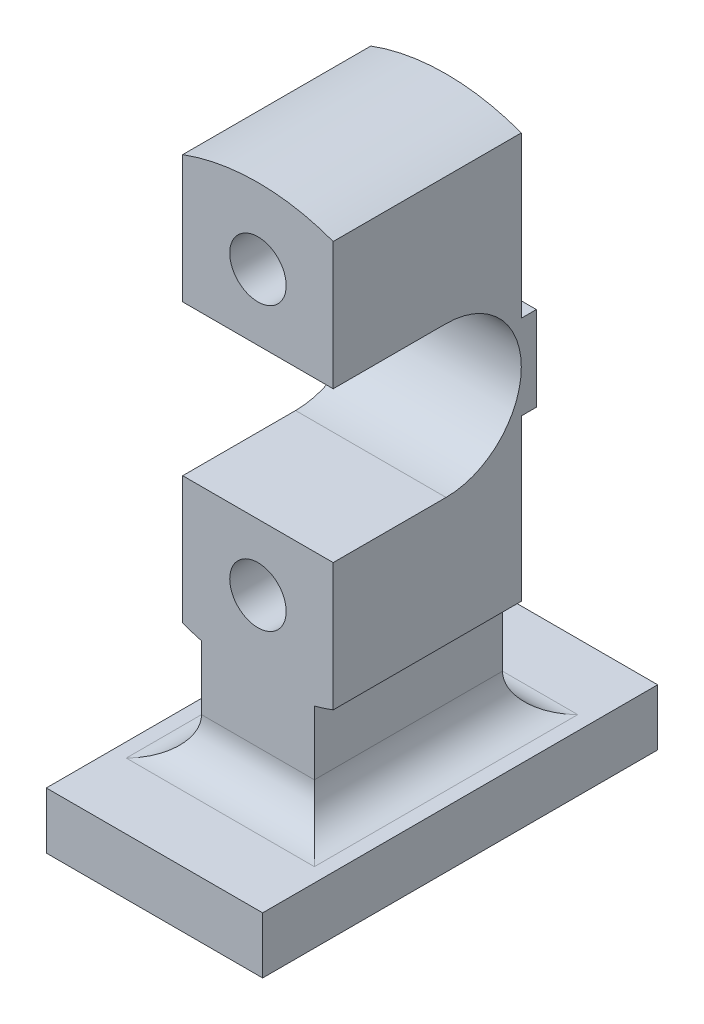
ISO-10303-21;
HEADER;
FILE_DESCRIPTION(('STEP AP214'),'2;1');
FILE_NAME('part.step','',(''),(''),'','','');
FILE_SCHEMA(('AUTOMOTIVE_DESIGN { 1 0 10303 214 1 1 1 1 }'));
ENDSEC;
DATA;
#1=APPLICATION_CONTEXT('core data for automotive mechanical design processes');
#2=APPLICATION_PROTOCOL_DEFINITION('international standard','automotive_design',2000,#1);
#3=PRODUCT_CONTEXT('',#1,'mechanical');
#4=PRODUCT('Part','Part','',(#3));
#5=PRODUCT_RELATED_PRODUCT_CATEGORY('part','',(#4));
#6=PRODUCT_DEFINITION_FORMATION('','',#4);
#7=PRODUCT_DEFINITION_CONTEXT('part definition',#1,'design');
#8=PRODUCT_DEFINITION('design','',#6,#7);
#9=PRODUCT_DEFINITION_SHAPE('','',#8);
#10=(LENGTH_UNIT() NAMED_UNIT(*) SI_UNIT(.MILLI.,.METRE.));
#11=(NAMED_UNIT(*) PLANE_ANGLE_UNIT() SI_UNIT($,.RADIAN.));
#12=(NAMED_UNIT(*) SI_UNIT($,.STERADIAN.) SOLID_ANGLE_UNIT());
#13=UNCERTAINTY_MEASURE_WITH_UNIT(LENGTH_MEASURE(1.E-05),#10,'distance_accuracy_value','');
#14=(GEOMETRIC_REPRESENTATION_CONTEXT(3) GLOBAL_UNCERTAINTY_ASSIGNED_CONTEXT((#13)) GLOBAL_UNIT_ASSIGNED_CONTEXT((#10,
#11,#12)) REPRESENTATION_CONTEXT('',''));
#15=CARTESIAN_POINT('',(0.,0.,0.));
#16=DIRECTION('',(0.,0.,1.));
#17=DIRECTION('',(1.,0.,0.));
#18=AXIS2_PLACEMENT_3D('',#15,#16,#17);
#19=CARTESIAN_POINT('',(0.,0.,50.));
#20=DIRECTION('',(0.,0.,-1.));
#21=DIRECTION('',(-1.,0.,0.));
#22=AXIS2_PLACEMENT_3D('',#19,#20,#21);
#23=PLANE('',#22);
#24=CARTESIAN_POINT('',(0.,-75.,50.));
#25=DIRECTION('',(0.,0.,1.));
#26=DIRECTION('',(-1.,0.,0.));
#27=AXIS2_PLACEMENT_3D('',#24,#25,#26);
#28=CIRCLE('',#27,15.);
#29=CARTESIAN_POINT('',(-15.,-75.,50.));
#30=VERTEX_POINT('',#29);
#31=EDGE_CURVE('E317',#30,#30,#28,.T.);
#32=ORIENTED_EDGE('',*,*,#31,.F.);
#33=EDGE_LOOP('',(#32));
#34=FACE_BOUND('',#33,.T.);
#35=DIRECTION('',(0.,1.,0.));
#36=VECTOR('',#35,1.);
#37=CARTESIAN_POINT('',(40.,-107.819293264239,50.));
#38=LINE('',#37,#36);
#39=CARTESIAN_POINT('',(40.,-107.819293264239,50.));
#40=VERTEX_POINT('',#39);
#41=CARTESIAN_POINT('',(40.,-40.,50.));
#42=VERTEX_POINT('',#41);
#43=EDGE_CURVE('E213',#40,#42,#38,.T.);
#44=ORIENTED_EDGE('',*,*,#43,.T.);
#45=DIRECTION('',(1.,0.,0.));
#46=VECTOR('',#45,1.);
#47=CARTESIAN_POINT('',(-168.062484748657,-40.,50.));
#48=LINE('',#47,#46);
#49=CARTESIAN_POINT('',(-40.,-40.,50.));
#50=VERTEX_POINT('',#49);
#51=EDGE_CURVE('E210',#50,#42,#48,.T.);
#52=ORIENTED_EDGE('',*,*,#51,.F.);
#53=DIRECTION('',(0.,-1.,0.));
#54=VECTOR('',#53,1.);
#55=CARTESIAN_POINT('',(-40.,-107.819293264239,50.));
#56=LINE('',#55,#54);
#57=CARTESIAN_POINT('',(-40.0000000000001,-107.819293264239,50.));
#58=VERTEX_POINT('',#57);
#59=EDGE_CURVE('E329',#50,#58,#56,.T.);
#60=ORIENTED_EDGE('',*,*,#59,.T.);
#61=CARTESIAN_POINT('',(0.,0.,50.));
#62=DIRECTION('',(0.,0.,1.));
#63=DIRECTION('',(1.,0.,0.));
#64=AXIS2_PLACEMENT_3D('',#61,#62,#63);
#65=CIRCLE('',#64,115.);
#66=CARTESIAN_POINT('',(-30.,-111.018016555873,50.));
#67=VERTEX_POINT('',#66);
#68=EDGE_CURVE('E335',#58,#67,#65,.T.);
#69=ORIENTED_EDGE('',*,*,#68,.T.);
#70=DIRECTION('',(0.,-1.,0.));
#71=VECTOR('',#70,1.);
#72=CARTESIAN_POINT('',(-30.,-111.018016555873,50.));
#73=LINE('',#72,#71);
#74=CARTESIAN_POINT('',(-30.,-145.,50.));
#75=VERTEX_POINT('',#74);
#76=EDGE_CURVE('E331',#67,#75,#73,.T.);
#77=ORIENTED_EDGE('',*,*,#76,.T.);
#78=DIRECTION('',(1.,0.,0.));
#79=VECTOR('',#78,1.);
#80=CARTESIAN_POINT('',(0.,-145.,50.));
#81=LINE('',#80,#79);
#82=CARTESIAN_POINT('',(30.,-145.,50.));
#83=VERTEX_POINT('',#82);
#84=EDGE_CURVE('E48',#75,#83,#81,.T.);
#85=ORIENTED_EDGE('',*,*,#84,.T.);
#86=DIRECTION('',(0.,1.,0.));
#87=VECTOR('',#86,1.);
#88=CARTESIAN_POINT('',(30.,-111.018016555873,50.));
#89=LINE('',#88,#87);
#90=CARTESIAN_POINT('',(30.,-111.018016555873,50.));
#91=VERTEX_POINT('',#90);
#92=EDGE_CURVE('E220',#83,#91,#89,.T.);
#93=ORIENTED_EDGE('',*,*,#92,.T.);
#94=CARTESIAN_POINT('',(0.,0.,50.));
#95=DIRECTION('',(0.,0.,1.));
#96=DIRECTION('',(1.,0.,0.));
#97=AXIS2_PLACEMENT_3D('',#94,#95,#96);
#98=CIRCLE('',#97,115.);
#99=EDGE_CURVE('E212',#91,#40,#98,.T.);
#100=ORIENTED_EDGE('',*,*,#99,.T.);
#101=EDGE_LOOP('',(#44,#52,#60,#69,#77,#85,#93,#100));
#102=FACE_BOUND('',#101,.T.);
#103=ADVANCED_FACE('F39',(#34,#102),#23,.F.);
#104=CARTESIAN_POINT('',(0.,0.,-50.));
#105=DIRECTION('',(0.,0.,-1.));
#106=DIRECTION('',(-1.,0.,0.));
#107=AXIS2_PLACEMENT_3D('',#104,#105,#106);
#108=PLANE('',#107);
#109=DIRECTION('',(1.,0.,0.));
#110=VECTOR('',#109,1.);
#111=CARTESIAN_POINT('',(-85.7055795281058,22.5,-50.));
#112=LINE('',#111,#110);
#113=CARTESIAN_POINT('',(-40.,22.5,-50.));
#114=VERTEX_POINT('',#113);
#115=CARTESIAN_POINT('',(40.,22.5,-50.));
#116=VERTEX_POINT('',#115);
#117=EDGE_CURVE('E409',#114,#116,#112,.T.);
#118=ORIENTED_EDGE('',*,*,#117,.F.);
#119=DIRECTION('',(0.,-1.,0.));
#120=VECTOR('',#119,1.);
#121=CARTESIAN_POINT('',(-40.,-107.819293264239,-50.));
#122=LINE('',#121,#120);
#123=CARTESIAN_POINT('',(-40.,107.819293264239,-50.));
#124=VERTEX_POINT('',#123);
#125=EDGE_CURVE('E227',#124,#114,#122,.T.);
#126=ORIENTED_EDGE('',*,*,#125,.F.);
#127=CARTESIAN_POINT('',(0.,0.,-50.));
#128=DIRECTION('',(0.,0.,1.));
#129=DIRECTION('',(-1.,0.,0.));
#130=AXIS2_PLACEMENT_3D('',#127,#128,#129);
#131=CIRCLE('',#130,115.);
#132=CARTESIAN_POINT('',(40.,107.819293264239,-50.));
#133=VERTEX_POINT('',#132);
#134=EDGE_CURVE('E222',#133,#124,#131,.T.);
#135=ORIENTED_EDGE('',*,*,#134,.F.);
#136=DIRECTION('',(0.,1.,0.));
#137=VECTOR('',#136,1.);
#138=CARTESIAN_POINT('',(40.,-107.819293264239,-50.));
#139=LINE('',#138,#137);
#140=EDGE_CURVE('E236',#116,#133,#139,.T.);
#141=ORIENTED_EDGE('',*,*,#140,.F.);
#142=EDGE_LOOP('',(#118,#126,#135,#141));
#143=FACE_BOUND('',#142,.T.);
#144=CARTESIAN_POINT('',(0.,75.,-50.));
#145=DIRECTION('',(0.,0.,1.));
#146=DIRECTION('',(1.,0.,0.));
#147=AXIS2_PLACEMENT_3D('',#144,#145,#146);
#148=CIRCLE('',#147,15.);
#149=CARTESIAN_POINT('',(15.,75.,-50.));
#150=VERTEX_POINT('',#149);
#151=EDGE_CURVE('E325',#150,#150,#148,.T.);
#152=ORIENTED_EDGE('',*,*,#151,.T.);
#153=EDGE_LOOP('',(#152));
#154=FACE_BOUND('',#153,.T.);
#155=ADVANCED_FACE('F450',(#143,#154),#108,.T.);
#156=CARTESIAN_POINT('',(-40.,107.819293264239,50.));
#157=VERTEX_POINT('',#156);
#158=CARTESIAN_POINT('',(-40.,40.,50.));
#159=VERTEX_POINT('',#158);
#160=EDGE_CURVE('E206',#157,#159,#56,.T.);
#161=ORIENTED_EDGE('',*,*,#160,.T.);
#162=DIRECTION('',(1.,0.,0.));
#163=VECTOR('',#162,1.);
#164=CARTESIAN_POINT('',(-168.062484748657,40.,50.));
#165=LINE('',#164,#163);
#166=CARTESIAN_POINT('',(40.,40.,50.));
#167=VERTEX_POINT('',#166);
#168=EDGE_CURVE('E192',#159,#167,#165,.T.);
#169=ORIENTED_EDGE('',*,*,#168,.T.);
#170=CARTESIAN_POINT('',(40.,107.819293264239,50.));
#171=VERTEX_POINT('',#170);
#172=EDGE_CURVE('E204',#167,#171,#38,.T.);
#173=ORIENTED_EDGE('',*,*,#172,.T.);
#174=CARTESIAN_POINT('',(0.,0.,50.));
#175=DIRECTION('',(0.,0.,1.));
#176=DIRECTION('',(-1.,0.,0.));
#177=AXIS2_PLACEMENT_3D('',#174,#175,#176);
#178=CIRCLE('',#177,115.);
#179=EDGE_CURVE('E244',#171,#157,#178,.T.);
#180=ORIENTED_EDGE('',*,*,#179,.T.);
#181=EDGE_LOOP('',(#161,#169,#173,#180));
#182=FACE_BOUND('',#181,.T.);
#183=CARTESIAN_POINT('',(0.,75.,50.));
#184=DIRECTION('',(0.,0.,1.));
#185=DIRECTION('',(1.,0.,0.));
#186=AXIS2_PLACEMENT_3D('',#183,#184,#185);
#187=CIRCLE('',#186,15.);
#188=CARTESIAN_POINT('',(15.,75.,50.));
#189=VERTEX_POINT('',#188);
#190=EDGE_CURVE('E223',#189,#189,#187,.T.);
#191=ORIENTED_EDGE('',*,*,#190,.F.);
#192=EDGE_LOOP('',(#191));
#193=FACE_BOUND('',#192,.T.);
#194=ADVANCED_FACE('F203',(#182,#193),#23,.F.);
#195=DIRECTION('',(1.,0.,0.));
#196=VECTOR('',#195,1.);
#197=CARTESIAN_POINT('',(-85.7055795281058,-22.5,-50.));
#198=LINE('',#197,#196);
#199=CARTESIAN_POINT('',(-40.,-22.5,-50.));
#200=VERTEX_POINT('',#199);
#201=CARTESIAN_POINT('',(40.,-22.5,-50.));
#202=VERTEX_POINT('',#201);
#203=EDGE_CURVE('E389',#200,#202,#198,.T.);
#204=ORIENTED_EDGE('',*,*,#203,.T.);
#205=CARTESIAN_POINT('',(40.,-107.819293264239,-50.));
#206=VERTEX_POINT('',#205);
#207=EDGE_CURVE('E239',#206,#202,#139,.T.);
#208=ORIENTED_EDGE('',*,*,#207,.F.);
#209=CARTESIAN_POINT('',(0.,0.,-50.));
#210=DIRECTION('',(0.,0.,1.));
#211=DIRECTION('',(1.,0.,0.));
#212=AXIS2_PLACEMENT_3D('',#209,#210,#211);
#213=CIRCLE('',#212,115.);
#214=CARTESIAN_POINT('',(30.,-111.018016555873,-50.));
#215=VERTEX_POINT('',#214);
#216=EDGE_CURVE('E237',#215,#206,#213,.T.);
#217=ORIENTED_EDGE('',*,*,#216,.F.);
#218=DIRECTION('',(0.,1.,0.));
#219=VECTOR('',#218,1.);
#220=CARTESIAN_POINT('',(30.,-111.018016555873,-50.));
#221=LINE('',#220,#219);
#222=CARTESIAN_POINT('',(30.,-145.,-50.));
#223=VERTEX_POINT('',#222);
#224=EDGE_CURVE('E235',#223,#215,#221,.T.);
#225=ORIENTED_EDGE('',*,*,#224,.F.);
#226=DIRECTION('',(1.,0.,0.));
#227=VECTOR('',#226,1.);
#228=CARTESIAN_POINT('',(-30.,-145.,-50.));
#229=LINE('',#228,#227);
#230=CARTESIAN_POINT('',(-30.,-145.,-50.));
#231=VERTEX_POINT('',#230);
#232=EDGE_CURVE('E268',#223,#231,#229,.F.);
#233=ORIENTED_EDGE('',*,*,#232,.T.);
#234=DIRECTION('',(0.,-1.,0.));
#235=VECTOR('',#234,1.);
#236=CARTESIAN_POINT('',(-30.,-111.018016555873,-50.));
#237=LINE('',#236,#235);
#238=CARTESIAN_POINT('',(-30.,-111.018016555873,-50.));
#239=VERTEX_POINT('',#238);
#240=EDGE_CURVE('E233',#239,#231,#237,.T.);
#241=ORIENTED_EDGE('',*,*,#240,.F.);
#242=CARTESIAN_POINT('',(0.,0.,-50.));
#243=DIRECTION('',(0.,0.,1.));
#244=DIRECTION('',(1.,0.,0.));
#245=AXIS2_PLACEMENT_3D('',#242,#243,#244);
#246=CIRCLE('',#245,115.);
#247=CARTESIAN_POINT('',(-40.0000000000001,-107.819293264239,-50.));
#248=VERTEX_POINT('',#247);
#249=EDGE_CURVE('E226',#248,#239,#246,.T.);
#250=ORIENTED_EDGE('',*,*,#249,.F.);
#251=EDGE_CURVE('E221',#200,#248,#122,.T.);
#252=ORIENTED_EDGE('',*,*,#251,.F.);
#253=EDGE_LOOP('',(#204,#208,#217,#225,#233,#241,#250,#252));
#254=FACE_BOUND('',#253,.T.);
#255=CARTESIAN_POINT('',(0.,-75.,-50.));
#256=DIRECTION('',(0.,0.,1.));
#257=DIRECTION('',(-1.,0.,0.));
#258=AXIS2_PLACEMENT_3D('',#255,#256,#257);
#259=CIRCLE('',#258,15.);
#260=CARTESIAN_POINT('',(-15.,-75.,-50.));
#261=VERTEX_POINT('',#260);
#262=EDGE_CURVE('E318',#261,#261,#259,.T.);
#263=ORIENTED_EDGE('',*,*,#262,.T.);
#264=EDGE_LOOP('',(#263));
#265=FACE_BOUND('',#264,.T.);
#266=ADVANCED_FACE('F378',(#254,#265),#108,.T.);
#267=CARTESIAN_POINT('',(0.,0.,50.));
#268=DIRECTION('',(0.,0.,-1.));
#269=DIRECTION('',(-1.,0.,0.));
#270=AXIS2_PLACEMENT_3D('',#267,#268,#269);
#271=CYLINDRICAL_SURFACE('',#270,115.);
#272=ORIENTED_EDGE('',*,*,#134,.T.);
#273=DIRECTION('',(0.,0.,-1.));
#274=VECTOR('',#273,1.);
#275=CARTESIAN_POINT('',(-40.,107.819293264239,50.));
#276=LINE('',#275,#274);
#277=EDGE_CURVE('E258',#157,#124,#276,.T.);
#278=ORIENTED_EDGE('',*,*,#277,.F.);
#279=ORIENTED_EDGE('',*,*,#179,.F.);
#280=DIRECTION('',(0.,0.,-1.));
#281=VECTOR('',#280,1.);
#282=CARTESIAN_POINT('',(40.,107.819293264239,50.));
#283=LINE('',#282,#281);
#284=EDGE_CURVE('E211',#171,#133,#283,.T.);
#285=ORIENTED_EDGE('',*,*,#284,.T.);
#286=EDGE_LOOP('',(#272,#278,#279,#285));
#287=FACE_BOUND('',#286,.T.);
#288=ADVANCED_FACE('F461',(#287),#271,.T.);
#289=CARTESIAN_POINT('',(-40.,-107.819293264239,50.));
#290=DIRECTION('',(1.,0.,0.));
#291=DIRECTION('',(0.,0.,-1.));
#292=AXIS2_PLACEMENT_3D('',#289,#290,#291);
#293=PLANE('',#292);
#294=ORIENTED_EDGE('',*,*,#59,.F.);
#295=DIRECTION('',(0.,0.,1.));
#296=VECTOR('',#295,1.);
#297=CARTESIAN_POINT('',(-40.,-40.,-10.));
#298=LINE('',#297,#296);
#299=CARTESIAN_POINT('',(-40.,-40.,-10.));
#300=VERTEX_POINT('',#299);
#301=EDGE_CURVE('E362',#300,#50,#298,.T.);
#302=ORIENTED_EDGE('',*,*,#301,.F.);
#303=CARTESIAN_POINT('',(-40.,0.,-9.99999999999999));
#304=DIRECTION('',(1.,0.,0.));
#305=DIRECTION('',(0.,0.,-1.));
#306=AXIS2_PLACEMENT_3D('',#303,#304,#305);
#307=CIRCLE('',#306,40.);
#308=CARTESIAN_POINT('',(-40.,40.,-10.));
#309=VERTEX_POINT('',#308);
#310=EDGE_CURVE('E396',#309,#300,#307,.F.);
#311=ORIENTED_EDGE('',*,*,#310,.F.);
#312=DIRECTION('',(0.,0.,-1.));
#313=VECTOR('',#312,1.);
#314=CARTESIAN_POINT('',(-40.,40.,-10.));
#315=LINE('',#314,#313);
#316=EDGE_CURVE('E399',#159,#309,#315,.T.);
#317=ORIENTED_EDGE('',*,*,#316,.F.);
#318=ORIENTED_EDGE('',*,*,#160,.F.);
#319=ORIENTED_EDGE('',*,*,#277,.T.);
#320=ORIENTED_EDGE('',*,*,#125,.T.);
#321=DIRECTION('',(0.,0.,-1.));
#322=VECTOR('',#321,1.);
#323=CARTESIAN_POINT('',(-40.,22.5,-50.));
#324=LINE('',#323,#322);
#325=CARTESIAN_POINT('',(-40.,22.5,-58.));
#326=VERTEX_POINT('',#325);
#327=EDGE_CURVE('E401',#114,#326,#324,.T.);
#328=ORIENTED_EDGE('',*,*,#327,.T.);
#329=DIRECTION('',(0.,-1.,0.));
#330=VECTOR('',#329,1.);
#331=CARTESIAN_POINT('',(-40.,22.5,-58.));
#332=LINE('',#331,#330);
#333=CARTESIAN_POINT('',(-40.,-22.5,-58.));
#334=VERTEX_POINT('',#333);
#335=EDGE_CURVE('E406',#326,#334,#332,.T.);
#336=ORIENTED_EDGE('',*,*,#335,.T.);
#337=DIRECTION('',(0.,0.,1.));
#338=VECTOR('',#337,1.);
#339=CARTESIAN_POINT('',(-40.,-22.5,-50.));
#340=LINE('',#339,#338);
#341=EDGE_CURVE('E280',#334,#200,#340,.T.);
#342=ORIENTED_EDGE('',*,*,#341,.T.);
#343=ORIENTED_EDGE('',*,*,#251,.T.);
#344=DIRECTION('',(0.,0.,-1.));
#345=VECTOR('',#344,1.);
#346=CARTESIAN_POINT('',(-40.0000000000001,-107.819293264239,50.));
#347=LINE('',#346,#345);
#348=EDGE_CURVE('E251',#58,#248,#347,.T.);
#349=ORIENTED_EDGE('',*,*,#348,.F.);
#350=EDGE_LOOP('',(#294,#302,#311,#317,#318,#319,#320,#328,#336,#342,#343,#349));
#351=FACE_BOUND('',#350,.T.);
#352=ADVANCED_FACE('F356',(#351),#293,.F.);
#353=CARTESIAN_POINT('',(0.,0.,50.));
#354=DIRECTION('',(0.,0.,-1.));
#355=DIRECTION('',(-1.,0.,0.));
#356=AXIS2_PLACEMENT_3D('',#353,#354,#355);
#357=CYLINDRICAL_SURFACE('',#356,115.);
#358=ORIENTED_EDGE('',*,*,#249,.T.);
#359=DIRECTION('',(0.,0.,-1.));
#360=VECTOR('',#359,1.);
#361=CARTESIAN_POINT('',(-30.,-111.018016555873,50.));
#362=LINE('',#361,#360);
#363=EDGE_CURVE('E246',#67,#239,#362,.T.);
#364=ORIENTED_EDGE('',*,*,#363,.F.);
#365=ORIENTED_EDGE('',*,*,#68,.F.);
#366=ORIENTED_EDGE('',*,*,#348,.T.);
#367=EDGE_LOOP('',(#358,#364,#365,#366));
#368=FACE_BOUND('',#367,.T.);
#369=ADVANCED_FACE('F366',(#368),#357,.T.);
#370=CARTESIAN_POINT('',(-30.,-111.018016555873,50.));
#371=DIRECTION('',(1.,0.,0.));
#372=DIRECTION('',(0.,1.,0.));
#373=AXIS2_PLACEMENT_3D('',#370,#371,#372);
#374=PLANE('',#373);
#375=ORIENTED_EDGE('',*,*,#240,.T.);
#376=DIRECTION('',(0.,0.,-1.));
#377=VECTOR('',#376,1.);
#378=CARTESIAN_POINT('',(-30.,-145.,50.));
#379=LINE('',#378,#377);
#380=EDGE_CURVE('E271',#231,#75,#379,.F.);
#381=ORIENTED_EDGE('',*,*,#380,.T.);
#382=ORIENTED_EDGE('',*,*,#76,.F.);
#383=ORIENTED_EDGE('',*,*,#363,.T.);
#384=EDGE_LOOP('',(#375,#381,#382,#383));
#385=FACE_BOUND('',#384,.T.);
#386=ADVANCED_FACE('F387',(#385),#374,.F.);
#387=CARTESIAN_POINT('',(30.,-111.018016555873,50.));
#388=DIRECTION('',(-1.,0.,0.));
#389=DIRECTION('',(0.,-1.,0.));
#390=AXIS2_PLACEMENT_3D('',#387,#388,#389);
#391=PLANE('',#390);
#392=ORIENTED_EDGE('',*,*,#92,.F.);
#393=DIRECTION('',(0.,0.,-1.));
#394=VECTOR('',#393,1.);
#395=CARTESIAN_POINT('',(30.,-145.,50.));
#396=LINE('',#395,#394);
#397=EDGE_CURVE('E11',#83,#223,#396,.T.);
#398=ORIENTED_EDGE('',*,*,#397,.T.);
#399=ORIENTED_EDGE('',*,*,#224,.T.);
#400=DIRECTION('',(0.,0.,-1.));
#401=VECTOR('',#400,1.);
#402=CARTESIAN_POINT('',(30.,-111.018016555873,50.));
#403=LINE('',#402,#401);
#404=EDGE_CURVE('E249',#91,#215,#403,.T.);
#405=ORIENTED_EDGE('',*,*,#404,.F.);
#406=EDGE_LOOP('',(#392,#398,#399,#405));
#407=FACE_BOUND('',#406,.T.);
#408=ADVANCED_FACE('F342',(#407),#391,.F.);
#409=CARTESIAN_POINT('',(0.,0.,50.));
#410=DIRECTION('',(0.,0.,-1.));
#411=DIRECTION('',(-1.,0.,0.));
#412=AXIS2_PLACEMENT_3D('',#409,#410,#411);
#413=CYLINDRICAL_SURFACE('',#412,115.);
#414=ORIENTED_EDGE('',*,*,#216,.T.);
#415=DIRECTION('',(0.,0.,-1.));
#416=VECTOR('',#415,1.);
#417=CARTESIAN_POINT('',(40.,-107.819293264239,50.));
#418=LINE('',#417,#416);
#419=EDGE_CURVE('E241',#40,#206,#418,.T.);
#420=ORIENTED_EDGE('',*,*,#419,.F.);
#421=ORIENTED_EDGE('',*,*,#99,.F.);
#422=ORIENTED_EDGE('',*,*,#404,.T.);
#423=EDGE_LOOP('',(#414,#420,#421,#422));
#424=FACE_BOUND('',#423,.T.);
#425=ADVANCED_FACE('F350',(#424),#413,.T.);
#426=CARTESIAN_POINT('',(40.,-107.819293264239,50.));
#427=DIRECTION('',(-1.,0.,0.));
#428=DIRECTION('',(0.,0.,1.));
#429=AXIS2_PLACEMENT_3D('',#426,#427,#428);
#430=PLANE('',#429);
#431=CARTESIAN_POINT('',(40.,0.,-9.99999999999999));
#432=DIRECTION('',(1.,0.,0.));
#433=DIRECTION('',(0.,0.,-1.));
#434=AXIS2_PLACEMENT_3D('',#431,#432,#433);
#435=CIRCLE('',#434,40.);
#436=CARTESIAN_POINT('',(40.,-40.,-10.));
#437=VERTEX_POINT('',#436);
#438=CARTESIAN_POINT('',(40.,40.,-9.99999999999999));
#439=VERTEX_POINT('',#438);
#440=EDGE_CURVE('E57',#437,#439,#435,.T.);
#441=ORIENTED_EDGE('',*,*,#440,.F.);
#442=DIRECTION('',(0.,0.,-1.));
#443=VECTOR('',#442,1.);
#444=CARTESIAN_POINT('',(40.,-40.,-10.));
#445=LINE('',#444,#443);
#446=EDGE_CURVE('E197',#42,#437,#445,.T.);
#447=ORIENTED_EDGE('',*,*,#446,.F.);
#448=ORIENTED_EDGE('',*,*,#43,.F.);
#449=ORIENTED_EDGE('',*,*,#419,.T.);
#450=ORIENTED_EDGE('',*,*,#207,.T.);
#451=DIRECTION('',(0.,0.,-1.));
#452=VECTOR('',#451,1.);
#453=CARTESIAN_POINT('',(40.,-22.5,-50.));
#454=LINE('',#453,#452);
#455=CARTESIAN_POINT('',(40.,-22.5,-58.));
#456=VERTEX_POINT('',#455);
#457=EDGE_CURVE('E391',#202,#456,#454,.T.);
#458=ORIENTED_EDGE('',*,*,#457,.T.);
#459=DIRECTION('',(0.,1.,0.));
#460=VECTOR('',#459,1.);
#461=CARTESIAN_POINT('',(40.,22.5,-58.));
#462=LINE('',#461,#460);
#463=CARTESIAN_POINT('',(40.,22.5,-58.));
#464=VERTEX_POINT('',#463);
#465=EDGE_CURVE('E398',#456,#464,#462,.T.);
#466=ORIENTED_EDGE('',*,*,#465,.T.);
#467=DIRECTION('',(0.,0.,1.));
#468=VECTOR('',#467,1.);
#469=CARTESIAN_POINT('',(40.,22.5,-50.));
#470=LINE('',#469,#468);
#471=EDGE_CURVE('E61',#464,#116,#470,.T.);
#472=ORIENTED_EDGE('',*,*,#471,.T.);
#473=ORIENTED_EDGE('',*,*,#140,.T.);
#474=ORIENTED_EDGE('',*,*,#284,.F.);
#475=ORIENTED_EDGE('',*,*,#172,.F.);
#476=DIRECTION('',(0.,0.,1.));
#477=VECTOR('',#476,1.);
#478=CARTESIAN_POINT('',(40.,40.,-10.));
#479=LINE('',#478,#477);
#480=EDGE_CURVE('E188',#439,#167,#479,.T.);
#481=ORIENTED_EDGE('',*,*,#480,.F.);
#482=EDGE_LOOP('',(#441,#447,#448,#449,#450,#458,#466,#472,#473,#474,#475,#481));
#483=FACE_BOUND('',#482,.T.);
#484=ADVANCED_FACE('F207',(#483),#430,.F.);
#485=CARTESIAN_POINT('',(0.,75.,50.));
#486=DIRECTION('',(0.,0.,-1.));
#487=DIRECTION('',(-1.,0.,0.));
#488=AXIS2_PLACEMENT_3D('',#485,#486,#487);
#489=CYLINDRICAL_SURFACE('',#488,15.);
#490=ORIENTED_EDGE('',*,*,#190,.T.);
#491=EDGE_LOOP('',(#490));
#492=FACE_BOUND('',#491,.T.);
#493=ORIENTED_EDGE('',*,*,#151,.F.);
#494=EDGE_LOOP('',(#493));
#495=FACE_BOUND('',#494,.T.);
#496=ADVANCED_FACE('F475',(#492,#495),#489,.F.);
#497=CARTESIAN_POINT('',(0.,-75.,50.));
#498=DIRECTION('',(0.,0.,-1.));
#499=DIRECTION('',(-1.,0.,0.));
#500=AXIS2_PLACEMENT_3D('',#497,#498,#499);
#501=CYLINDRICAL_SURFACE('',#500,15.);
#502=ORIENTED_EDGE('',*,*,#31,.T.);
#503=EDGE_LOOP('',(#502));
#504=FACE_BOUND('',#503,.T.);
#505=ORIENTED_EDGE('',*,*,#262,.F.);
#506=EDGE_LOOP('',(#505));
#507=FACE_BOUND('',#506,.T.);
#508=ADVANCED_FACE('F619',(#504,#507),#501,.F.);
#509=CARTESIAN_POINT('',(57.5,-195.,-105.));
#510=DIRECTION('',(-1.,0.,0.));
#511=DIRECTION('',(0.,0.,1.));
#512=AXIS2_PLACEMENT_3D('',#509,#510,#511);
#513=PLANE('',#512);
#514=DIRECTION('',(0.,0.,1.));
#515=VECTOR('',#514,1.);
#516=CARTESIAN_POINT('',(57.5,-165.,-105.));
#517=LINE('',#516,#515);
#518=CARTESIAN_POINT('',(57.5,-165.,-105.));
#519=VERTEX_POINT('',#518);
#520=CARTESIAN_POINT('',(57.5,-165.,105.));
#521=VERTEX_POINT('',#520);
#522=EDGE_CURVE('E283',#519,#521,#517,.T.);
#523=ORIENTED_EDGE('',*,*,#522,.T.);
#524=DIRECTION('',(0.,1.,0.));
#525=VECTOR('',#524,1.);
#526=CARTESIAN_POINT('',(57.5,-195.,105.));
#527=LINE('',#526,#525);
#528=CARTESIAN_POINT('',(57.5,-195.,105.));
#529=VERTEX_POINT('',#528);
#530=EDGE_CURVE('E312',#529,#521,#527,.T.);
#531=ORIENTED_EDGE('',*,*,#530,.F.);
#532=DIRECTION('',(0.,0.,1.));
#533=VECTOR('',#532,1.);
#534=CARTESIAN_POINT('',(57.5,-195.,-105.));
#535=LINE('',#534,#533);
#536=CARTESIAN_POINT('',(57.5,-195.,-105.));
#537=VERTEX_POINT('',#536);
#538=EDGE_CURVE('E308',#537,#529,#535,.T.);
#539=ORIENTED_EDGE('',*,*,#538,.F.);
#540=DIRECTION('',(0.,1.,0.));
#541=VECTOR('',#540,1.);
#542=CARTESIAN_POINT('',(57.5,-195.,-105.));
#543=LINE('',#542,#541);
#544=EDGE_CURVE('E307',#537,#519,#543,.T.);
#545=ORIENTED_EDGE('',*,*,#544,.T.);
#546=EDGE_LOOP('',(#523,#531,#539,#545));
#547=FACE_BOUND('',#546,.T.);
#548=ADVANCED_FACE('F428',(#547),#513,.F.);
#549=CARTESIAN_POINT('',(-57.5,-195.,105.));
#550=DIRECTION('',(0.,0.,-1.));
#551=DIRECTION('',(-1.,0.,0.));
#552=AXIS2_PLACEMENT_3D('',#549,#550,#551);
#553=PLANE('',#552);
#554=DIRECTION('',(-1.,0.,0.));
#555=VECTOR('',#554,1.);
#556=CARTESIAN_POINT('',(-57.5,-165.,105.));
#557=LINE('',#556,#555);
#558=CARTESIAN_POINT('',(-57.5,-165.,105.));
#559=VERTEX_POINT('',#558);
#560=EDGE_CURVE('E292',#521,#559,#557,.T.);
#561=ORIENTED_EDGE('',*,*,#560,.T.);
#562=DIRECTION('',(0.,1.,0.));
#563=VECTOR('',#562,1.);
#564=CARTESIAN_POINT('',(-57.5,-195.,105.));
#565=LINE('',#564,#563);
#566=CARTESIAN_POINT('',(-57.5,-195.,105.));
#567=VERTEX_POINT('',#566);
#568=EDGE_CURVE('E315',#567,#559,#565,.T.);
#569=ORIENTED_EDGE('',*,*,#568,.F.);
#570=DIRECTION('',(-1.,0.,0.));
#571=VECTOR('',#570,1.);
#572=CARTESIAN_POINT('',(-57.5,-195.,105.));
#573=LINE('',#572,#571);
#574=EDGE_CURVE('E418',#529,#567,#573,.T.);
#575=ORIENTED_EDGE('',*,*,#574,.F.);
#576=ORIENTED_EDGE('',*,*,#530,.T.);
#577=EDGE_LOOP('',(#561,#569,#575,#576));
#578=FACE_BOUND('',#577,.T.);
#579=ADVANCED_FACE('F429',(#578),#553,.F.);
#580=CARTESIAN_POINT('',(-57.5,-195.,-105.));
#581=DIRECTION('',(1.,0.,0.));
#582=DIRECTION('',(0.,0.,-1.));
#583=AXIS2_PLACEMENT_3D('',#580,#581,#582);
#584=PLANE('',#583);
#585=DIRECTION('',(0.,0.,-1.));
#586=VECTOR('',#585,1.);
#587=CARTESIAN_POINT('',(-57.5,-165.,-105.));
#588=LINE('',#587,#586);
#589=CARTESIAN_POINT('',(-57.5,-165.,-105.));
#590=VERTEX_POINT('',#589);
#591=EDGE_CURVE('E299',#559,#590,#588,.T.);
#592=ORIENTED_EDGE('',*,*,#591,.T.);
#593=DIRECTION('',(0.,1.,0.));
#594=VECTOR('',#593,1.);
#595=CARTESIAN_POINT('',(-57.5,-195.,-105.));
#596=LINE('',#595,#594);
#597=CARTESIAN_POINT('',(-57.5,-195.,-105.));
#598=VERTEX_POINT('',#597);
#599=EDGE_CURVE('E310',#598,#590,#596,.T.);
#600=ORIENTED_EDGE('',*,*,#599,.F.);
#601=DIRECTION('',(0.,0.,-1.));
#602=VECTOR('',#601,1.);
#603=CARTESIAN_POINT('',(-57.5,-195.,-105.));
#604=LINE('',#603,#602);
#605=EDGE_CURVE('E417',#567,#598,#604,.T.);
#606=ORIENTED_EDGE('',*,*,#605,.F.);
#607=ORIENTED_EDGE('',*,*,#568,.T.);
#608=EDGE_LOOP('',(#592,#600,#606,#607));
#609=FACE_BOUND('',#608,.T.);
#610=ADVANCED_FACE('F432',(#609),#584,.F.);
#611=CARTESIAN_POINT('',(-57.5,-195.,-105.));
#612=DIRECTION('',(0.,0.,1.));
#613=DIRECTION('',(1.,0.,0.));
#614=AXIS2_PLACEMENT_3D('',#611,#612,#613);
#615=PLANE('',#614);
#616=DIRECTION('',(1.,0.,0.));
#617=VECTOR('',#616,1.);
#618=CARTESIAN_POINT('',(-57.5,-165.,-105.));
#619=LINE('',#618,#617);
#620=EDGE_CURVE('E305',#590,#519,#619,.T.);
#621=ORIENTED_EDGE('',*,*,#620,.T.);
#622=ORIENTED_EDGE('',*,*,#544,.F.);
#623=DIRECTION('',(1.,0.,0.));
#624=VECTOR('',#623,1.);
#625=CARTESIAN_POINT('',(-57.5,-195.,-105.));
#626=LINE('',#625,#624);
#627=EDGE_CURVE('E298',#598,#537,#626,.T.);
#628=ORIENTED_EDGE('',*,*,#627,.F.);
#629=ORIENTED_EDGE('',*,*,#599,.T.);
#630=EDGE_LOOP('',(#621,#622,#628,#629));
#631=FACE_BOUND('',#630,.T.);
#632=ADVANCED_FACE('F426',(#631),#615,.F.);
#633=CARTESIAN_POINT('',(0.,-195.,0.));
#634=DIRECTION('',(0.,1.,0.));
#635=DIRECTION('',(0.,0.,1.));
#636=AXIS2_PLACEMENT_3D('',#633,#634,#635);
#637=PLANE('',#636);
#638=ORIENTED_EDGE('',*,*,#538,.T.);
#639=ORIENTED_EDGE('',*,*,#574,.T.);
#640=ORIENTED_EDGE('',*,*,#605,.T.);
#641=ORIENTED_EDGE('',*,*,#627,.T.);
#642=EDGE_LOOP('',(#638,#639,#640,#641));
#643=FACE_BOUND('',#642,.T.);
#644=ADVANCED_FACE('F421',(#643),#637,.F.);
#645=CARTESIAN_POINT('',(0.,-165.,0.));
#646=DIRECTION('',(0.,1.,0.));
#647=DIRECTION('',(0.,0.,1.));
#648=AXIS2_PLACEMENT_3D('',#645,#646,#647);
#649=PLANE('',#648);
#650=DIRECTION('',(0.,0.,-1.));
#651=VECTOR('',#650,1.);
#652=CARTESIAN_POINT('',(-50.,-165.,0.));
#653=LINE('',#652,#651);
#654=CARTESIAN_POINT('',(-50.,-165.,70.));
#655=VERTEX_POINT('',#654);
#656=CARTESIAN_POINT('',(-50.,-165.,-70.));
#657=VERTEX_POINT('',#656);
#658=EDGE_CURVE('E263',#655,#657,#653,.T.);
#659=ORIENTED_EDGE('',*,*,#658,.T.);
#660=DIRECTION('',(1.,0.,0.));
#661=VECTOR('',#660,1.);
#662=CARTESIAN_POINT('',(30.,-165.,-70.));
#663=LINE('',#662,#661);
#664=CARTESIAN_POINT('',(50.,-165.,-70.));
#665=VERTEX_POINT('',#664);
#666=EDGE_CURVE('E264',#657,#665,#663,.T.);
#667=ORIENTED_EDGE('',*,*,#666,.T.);
#668=DIRECTION('',(0.,0.,-1.));
#669=VECTOR('',#668,1.);
#670=CARTESIAN_POINT('',(50.,-165.,0.));
#671=LINE('',#670,#669);
#672=CARTESIAN_POINT('',(50.,-165.,70.));
#673=VERTEX_POINT('',#672);
#674=EDGE_CURVE('E259',#665,#673,#671,.F.);
#675=ORIENTED_EDGE('',*,*,#674,.T.);
#676=DIRECTION('',(1.,0.,0.));
#677=VECTOR('',#676,1.);
#678=CARTESIAN_POINT('',(0.,-165.,70.));
#679=LINE('',#678,#677);
#680=EDGE_CURVE('E261',#673,#655,#679,.F.);
#681=ORIENTED_EDGE('',*,*,#680,.T.);
#682=EDGE_LOOP('',(#659,#667,#675,#681));
#683=FACE_BOUND('',#682,.T.);
#684=ORIENTED_EDGE('',*,*,#522,.F.);
#685=ORIENTED_EDGE('',*,*,#620,.F.);
#686=ORIENTED_EDGE('',*,*,#591,.F.);
#687=ORIENTED_EDGE('',*,*,#560,.F.);
#688=EDGE_LOOP('',(#684,#685,#686,#687));
#689=FACE_BOUND('',#688,.T.);
#690=ADVANCED_FACE('F436',(#683,#689),#649,.T.);
#691=CARTESIAN_POINT('',(0.,-145.,70.));
#692=DIRECTION('',(1.,0.,0.));
#693=DIRECTION('',(0.,0.,-1.));
#694=AXIS2_PLACEMENT_3D('',#691,#692,#693);
#695=CYLINDRICAL_SURFACE('',#694,20.);
#696=CARTESIAN_POINT('',(50.,-145.,70.));
#697=DIRECTION('',(0.707106781186547,0.,-0.707106781186547));
#698=DIRECTION('',(-0.707106781186547,0.,-0.707106781186547));
#699=AXIS2_PLACEMENT_3D('',#696,#697,#698);
#700=ELLIPSE('',#699,28.2842712474619,20.);
#701=EDGE_CURVE('E279',#83,#673,#700,.F.);
#702=ORIENTED_EDGE('',*,*,#701,.F.);
#703=ORIENTED_EDGE('',*,*,#84,.F.);
#704=CARTESIAN_POINT('',(-50.,-145.,70.));
#705=DIRECTION('',(0.707106781186547,0.,0.707106781186547));
#706=DIRECTION('',(0.707106781186547,0.,-0.707106781186547));
#707=AXIS2_PLACEMENT_3D('',#704,#705,#706);
#708=ELLIPSE('',#707,28.2842712474619,20.);
#709=EDGE_CURVE('E43',#655,#75,#708,.T.);
#710=ORIENTED_EDGE('',*,*,#709,.F.);
#711=ORIENTED_EDGE('',*,*,#680,.F.);
#712=EDGE_LOOP('',(#702,#703,#710,#711));
#713=FACE_BOUND('',#712,.T.);
#714=ADVANCED_FACE('F41',(#713),#695,.F.);
#715=CARTESIAN_POINT('',(-50.,-145.,0.));
#716=DIRECTION('',(0.,0.,-1.));
#717=DIRECTION('',(-1.,0.,0.));
#718=AXIS2_PLACEMENT_3D('',#715,#716,#717);
#719=CYLINDRICAL_SURFACE('',#718,20.);
#720=ORIENTED_EDGE('',*,*,#709,.T.);
#721=ORIENTED_EDGE('',*,*,#380,.F.);
#722=CARTESIAN_POINT('',(-50.,-145.,-70.));
#723=DIRECTION('',(0.707106781186547,0.,-0.707106781186547));
#724=DIRECTION('',(-0.707106781186547,0.,-0.707106781186547));
#725=AXIS2_PLACEMENT_3D('',#722,#723,#724);
#726=ELLIPSE('',#725,28.2842712474619,20.);
#727=EDGE_CURVE('E277',#657,#231,#726,.F.);
#728=ORIENTED_EDGE('',*,*,#727,.F.);
#729=ORIENTED_EDGE('',*,*,#658,.F.);
#730=EDGE_LOOP('',(#720,#721,#728,#729));
#731=FACE_BOUND('',#730,.T.);
#732=ADVANCED_FACE('F384',(#731),#719,.F.);
#733=CARTESIAN_POINT('',(50.,-145.,50.));
#734=DIRECTION('',(0.,0.,-1.));
#735=DIRECTION('',(-1.,0.,0.));
#736=AXIS2_PLACEMENT_3D('',#733,#734,#735);
#737=CYLINDRICAL_SURFACE('',#736,20.);
#738=ORIENTED_EDGE('',*,*,#701,.T.);
#739=ORIENTED_EDGE('',*,*,#674,.F.);
#740=CARTESIAN_POINT('',(50.,-145.,-70.));
#741=DIRECTION('',(-0.707106781186547,0.,-0.707106781186547));
#742=DIRECTION('',(0.707106781186547,0.,-0.707106781186547));
#743=AXIS2_PLACEMENT_3D('',#740,#741,#742);
#744=ELLIPSE('',#743,28.2842712474619,20.);
#745=EDGE_CURVE('E273',#223,#665,#744,.F.);
#746=ORIENTED_EDGE('',*,*,#745,.F.);
#747=ORIENTED_EDGE('',*,*,#397,.F.);
#748=EDGE_LOOP('',(#738,#739,#746,#747));
#749=FACE_BOUND('',#748,.T.);
#750=ADVANCED_FACE('F372',(#749),#737,.F.);
#751=CARTESIAN_POINT('',(0.,-145.,-70.));
#752=DIRECTION('',(-1.,0.,0.));
#753=DIRECTION('',(0.,0.,1.));
#754=AXIS2_PLACEMENT_3D('',#751,#752,#753);
#755=CYLINDRICAL_SURFACE('',#754,20.);
#756=ORIENTED_EDGE('',*,*,#727,.T.);
#757=ORIENTED_EDGE('',*,*,#232,.F.);
#758=ORIENTED_EDGE('',*,*,#745,.T.);
#759=ORIENTED_EDGE('',*,*,#666,.F.);
#760=EDGE_LOOP('',(#756,#757,#758,#759));
#761=FACE_BOUND('',#760,.T.);
#762=ADVANCED_FACE('F385',(#761),#755,.F.);
#763=CARTESIAN_POINT('',(-85.7055795281058,22.5,-50.));
#764=DIRECTION('',(0.,1.,0.));
#765=DIRECTION('',(0.,0.,1.));
#766=AXIS2_PLACEMENT_3D('',#763,#764,#765);
#767=PLANE('',#766);
#768=ORIENTED_EDGE('',*,*,#327,.F.);
#769=ORIENTED_EDGE('',*,*,#117,.T.);
#770=ORIENTED_EDGE('',*,*,#471,.F.);
#771=DIRECTION('',(1.,0.,0.));
#772=VECTOR('',#771,1.);
#773=CARTESIAN_POINT('',(-85.7055795281058,22.5,-58.));
#774=LINE('',#773,#772);
#775=EDGE_CURVE('E408',#326,#464,#774,.T.);
#776=ORIENTED_EDGE('',*,*,#775,.F.);
#777=EDGE_LOOP('',(#768,#769,#770,#776));
#778=FACE_BOUND('',#777,.T.);
#779=ADVANCED_FACE('F484',(#778),#767,.T.);
#780=CARTESIAN_POINT('',(-85.7055795281058,22.5,-58.));
#781=DIRECTION('',(0.,0.,-1.));
#782=DIRECTION('',(-1.,0.,0.));
#783=AXIS2_PLACEMENT_3D('',#780,#781,#782);
#784=PLANE('',#783);
#785=ORIENTED_EDGE('',*,*,#335,.F.);
#786=ORIENTED_EDGE('',*,*,#775,.T.);
#787=ORIENTED_EDGE('',*,*,#465,.F.);
#788=DIRECTION('',(1.,0.,0.));
#789=VECTOR('',#788,1.);
#790=CARTESIAN_POINT('',(-85.7055795281058,-22.5,-58.));
#791=LINE('',#790,#789);
#792=EDGE_CURVE('E392',#334,#456,#791,.T.);
#793=ORIENTED_EDGE('',*,*,#792,.F.);
#794=EDGE_LOOP('',(#785,#786,#787,#793));
#795=FACE_BOUND('',#794,.T.);
#796=ADVANCED_FACE('F519',(#795),#784,.T.);
#797=CARTESIAN_POINT('',(-85.7055795281058,-22.5,-50.));
#798=DIRECTION('',(0.,-1.,0.));
#799=DIRECTION('',(0.,0.,-1.));
#800=AXIS2_PLACEMENT_3D('',#797,#798,#799);
#801=PLANE('',#800);
#802=ORIENTED_EDGE('',*,*,#341,.F.);
#803=ORIENTED_EDGE('',*,*,#792,.T.);
#804=ORIENTED_EDGE('',*,*,#457,.F.);
#805=ORIENTED_EDGE('',*,*,#203,.F.);
#806=EDGE_LOOP('',(#802,#803,#804,#805));
#807=FACE_BOUND('',#806,.T.);
#808=ADVANCED_FACE('F527',(#807),#801,.T.);
#809=CARTESIAN_POINT('',(-168.062484748657,0.,-9.99999999999999));
#810=DIRECTION('',(1.,0.,0.));
#811=DIRECTION('',(0.,0.,-1.));
#812=AXIS2_PLACEMENT_3D('',#809,#810,#811);
#813=CYLINDRICAL_SURFACE('',#812,40.);
#814=ORIENTED_EDGE('',*,*,#310,.T.);
#815=DIRECTION('',(1.,0.,0.));
#816=VECTOR('',#815,1.);
#817=CARTESIAN_POINT('',(-168.062484748657,-40.,-10.));
#818=LINE('',#817,#816);
#819=EDGE_CURVE('E358',#300,#437,#818,.T.);
#820=ORIENTED_EDGE('',*,*,#819,.T.);
#821=ORIENTED_EDGE('',*,*,#440,.T.);
#822=DIRECTION('',(1.,0.,0.));
#823=VECTOR('',#822,1.);
#824=CARTESIAN_POINT('',(-168.062484748657,40.,-10.));
#825=LINE('',#824,#823);
#826=EDGE_CURVE('E191',#309,#439,#825,.T.);
#827=ORIENTED_EDGE('',*,*,#826,.F.);
#828=EDGE_LOOP('',(#814,#820,#821,#827));
#829=FACE_BOUND('',#828,.T.);
#830=ADVANCED_FACE('F534',(#829),#813,.F.);
#831=CARTESIAN_POINT('',(-168.062484748657,-40.,-10.));
#832=DIRECTION('',(0.,-1.,0.));
#833=DIRECTION('',(0.,0.,-1.));
#834=AXIS2_PLACEMENT_3D('',#831,#832,#833);
#835=PLANE('',#834);
#836=ORIENTED_EDGE('',*,*,#301,.T.);
#837=ORIENTED_EDGE('',*,*,#51,.T.);
#838=ORIENTED_EDGE('',*,*,#446,.T.);
#839=ORIENTED_EDGE('',*,*,#819,.F.);
#840=EDGE_LOOP('',(#836,#837,#838,#839));
#841=FACE_BOUND('',#840,.T.);
#842=ADVANCED_FACE('F550',(#841),#835,.F.);
#843=CARTESIAN_POINT('',(-168.062484748657,40.,-10.));
#844=DIRECTION('',(0.,1.,0.));
#845=DIRECTION('',(0.,0.,1.));
#846=AXIS2_PLACEMENT_3D('',#843,#844,#845);
#847=PLANE('',#846);
#848=ORIENTED_EDGE('',*,*,#316,.T.);
#849=ORIENTED_EDGE('',*,*,#826,.T.);
#850=ORIENTED_EDGE('',*,*,#480,.T.);
#851=ORIENTED_EDGE('',*,*,#168,.F.);
#852=EDGE_LOOP('',(#848,#849,#850,#851));
#853=FACE_BOUND('',#852,.T.);
#854=ADVANCED_FACE('F194',(#853),#847,.F.);
#855=CLOSED_SHELL('',(#103,#155,#194,#266,#288,#352,#369,#386,#408,#425,#484,#496,#508,#548,
#579,#610,#632,#644,#690,#714,#732,#750,#762,#779,#796,#808,#830,#842,#854));
#856=MANIFOLD_SOLID_BREP('B2',#855);
#857=ADVANCED_BREP_SHAPE_REPRESENTATION('',(#18,#856),#14);
#858=SHAPE_DEFINITION_REPRESENTATION(#9,#857);
ENDSEC;
END-ISO-10303-21;
